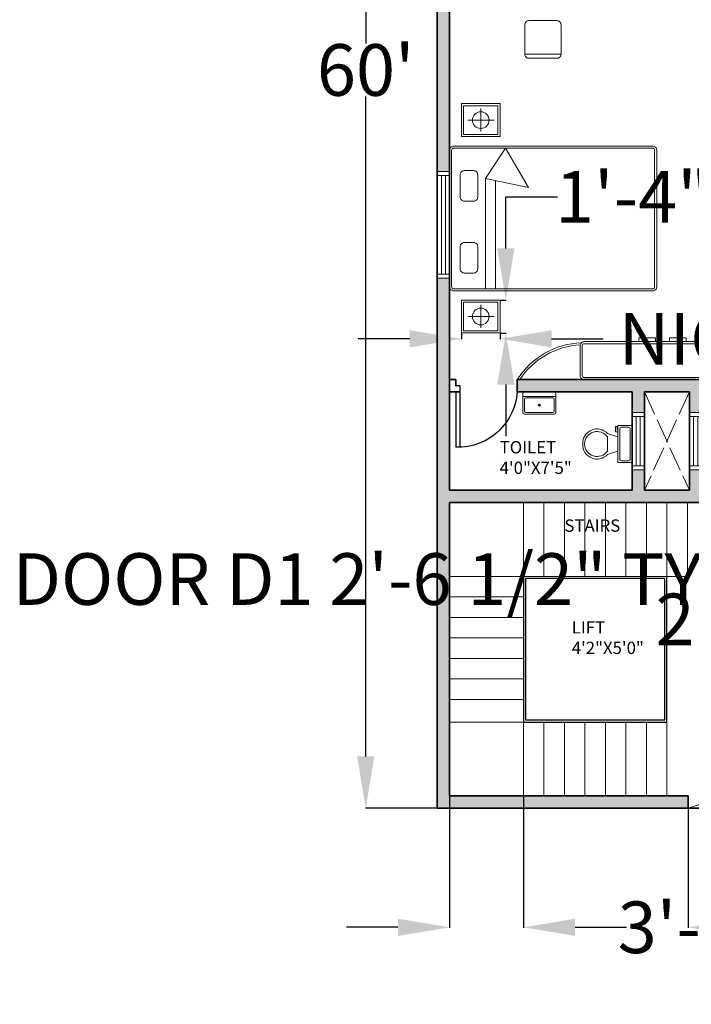
# Model space of a CAD drawing. Units: inches. Extents: x 35 to 5908, y 4 to 3165.
# Tile 1 of 6: x 4845 to 5173, y 2226 to 2706. Entities that reach past the tile are written whole.
import ezdxf

# ---------------------------------------------------------------- set-up
doc = ezdxf.new("R2010")
doc.units = ezdxf.units.IN
doc.header["$MEASUREMENT"] = 0
doc.linetypes.add('ACAD_ISO02W100', pattern=[15, 12, -3])
for name, color, linetype, lineweight in [('A-ANNO-DIMS', 2, 'Continuous', 18), ('A-ANNO-SYMB', 7, 'Continuous', 18), ('A-DOOR', 4, 'Continuous', 25), ('A-FLOR-CASE', 8, 'Continuous', 18), ('A-FLOR-EVTR', 7, 'Continuous', 25), ('A-FLOR-FIXT', 8, 'Continuous', 18), ('A-FLOR-SHFT', 8, 'ACAD_ISO02W100', 13), ('A-FLOR-STRS', 7, 'Continuous', 18), ('A-FURN', 8, 'Continuous', 18), ('A-WALL', 7, 'Continuous', 35), ('A-WALL-PATT', 252, 'Continuous', 13)]:
    doc.layers.add(name, color=color, linetype=linetype, lineweight=lineweight)
doc.layers.add('A-AREA-IDEN', color=30, linetype='Continuous', lineweight=18, true_color=0xf8991e)
doc.layers.add('A-GLAZ', color=30, linetype='Continuous', lineweight=18, true_color=0xf8991e)
doc.styles.get("Standard").update_dxf_attribs({"font": 'arial.ttf'})
doc.dimstyles.get("Standard").update_dxf_attribs({"dimtxt": 25.18, "dimasz": 25.18, "dimexe": 0.18, "dimexo": 0.0625, "dimgap": 0.09, "dimtad": 0, "dimtih": 1, "dimtoh": 1, "dimdec": 0, "dimzin": 0, "dimdsep": 46, "dimlunit": 3, "dimtxsty": 'Standard', "dimcen": 0.09, "dimadec": 0, "dimazin": 0, "dimtfac": 1, "dimtdec": 0, "dimtofl": 0, "dimtmove": 0, "dimatfit": 3, "dimfxl": 1, "dimtolj": 1, "dimtzin": 0, "dimarcsym": 0})

# ---------------------------------------------------------------- blocks, each defined once
blk = doc.blocks.new('Sink-single - 30 in top')
blk.add_line((-15, -3.999996), (15, -3.999996))
for points in [[(-13.5, 0), (13.5, 0)], [(-15, -18.499996), (-15, -1.5)], [(-13.5, -17.499996), (-13.5, -6.499996)], [(-12.5, -5.499996), (12.5, -5.499996)], [(13.5, -6.499996), (13.5, -17.499996)], [(15, -1.5), (15, -18.499996)], [(13.5, -19.999996), (-13.5, -19.999996)], [(12.5, -18.499996), (-12.5, -18.499996)]]:
    blk.add_lwpolyline(points)
for radius in [1, 0.5]:
    blk.add_circle((0, -11.999996), radius)
for centre, radius, start, end in [((-13.5, -1.5), 1.5, 90, 180), ((-12.5, -6.499996), 1, 90, 180), ((12.5, -6.499996), 1, 0, 90), ((13.5, -1.5), 1.5, 0, 90), ((-12.5, -17.499996), 1, 180, 270), ((12.5, -17.499996), 1, 270, 0), ((-13.5, -18.499996), 1.5, 180, 270), ((13.5, -18.499996), 1.5, 270, 0)]:
    blk.add_arc(centre, radius, start, end)
blk = doc.blocks.new('*U4')
for p, q in [((9.5, -6), (9.5, -2)), ((-10, -8.5), (-8, -8.5)), ((-10, -9.5), (-10, -8.5)), ((-7, -9.5), (-10, -9.5)), ((-8, -8.5), (-8, -8)), ((-7, -8), (-7, -9.5)), ((-4, -8), (-6, -14)), ((4, -8), (6, -14)), ((4, -14), (-4, -14))]:
    blk.add_line(p, q)
blk.add_lwpolyline([(10.5, -8), (10.5, 0), (-10.5, 0), (-10.5, -8)], close=True)
for points in [[(-9.5, -2), (-9.5, -6)], [(8.5, -1), (-8.5, -1)], [(-8.5, -7), (8.5, -7)]]:
    blk.add_lwpolyline(points)
for centre, radius, start, end in [((-8.625, -1.875), 0.8839, 81.8699, 188.1301), ((8.625, -1.875), 0.8839, 351.8699, 98.1301), ((-8.625, -6.125), 0.8839, 171.869898, 278.1301), ((8.625, -6.125), 0.8839, 261.8699, 8.1301), ((-0.4772, -19.9188), 8.0953, 133.01722, 273.38), ((0.0374, -19.8731), 7.127, 124.50543, 269.7), ((-0.0373, -19.8731), 7.127, 270.3, 55.4946), ((0.4773, -19.9188), 8.0953, 266.62, 46.9828)]:
    blk.add_arc(centre, radius, start, end)
blk = doc.blocks.new('*D7')
at = {"layer": 'A-ANNO-DIMS', "color": 0, "lineweight": -2, "transparency": 16777216}
for p, q in [((5048.73, 3041.84), (5013.71, 3041.84)), ((5013.89, 3016.66), (5013.89, 2694.76)), ((5013.89, 2346.96), (5013.89, 2668.86)), ((5048.73, 2321.78), (5013.71, 2321.78))]:
    blk.add_line(p, q, dxfattribs=at)
for points in [[(5009.69, 3016.66), (5018.09, 3016.66), (5013.89, 3041.84)], [(5009.69, 2346.96), (5018.09, 2346.96), (5013.89, 2321.78)]]:
    blk.add_solid(points, dxfattribs=at)
at = {"layer": 'Defpoints', "color": 0, "lineweight": -2, "transparency": 16777216}
for p in [(5048.79, 3041.84), (5013.89, 2321.78), (5048.79, 2321.78)]:
    blk.add_point(p, dxfattribs=at)
at = {"layer": 'A-ANNO-DIMS', "color": 0, "transparency": 16777216, "insert": (5013.89, 2681.81), "char_height": 25.18, "attachment_point": 5}
blk.add_mtext("\\A1;60'", dxfattribs=at)
blk = doc.blocks.new('DOOR-30-3-JAMB')
for p, q in [((-2, -27), (-2, 0)), ((0, -30), (0, 0)), ((0, -30), (-2, -30))]:
    blk.add_line(p, q)
blk.add_arc((-1, -29), 29.02, 358.0251, 91.9749)
blk = doc.blocks.new('WINDOW-48')
for p, q in [((0, 0), (0, 6)), ((2, 0), (2, 6)), ((50, 0), (50, 6)), ((52, 0), (52, 6)), ((2, 4), (50, 4)), ((2, 2), (50, 2))]:
    blk.add_line(p, q)
blk = doc.blocks.new('WINDOW-24')
for p, q in [((0, 0), (0, 6)), ((2, 0), (2, 6)), ((26, 0), (26, 6)), ((28, 0), (28, 6)), ((2, 4), (26, 4)), ((2, 2), (26, 2))]:
    blk.add_line(p, q)
blk = doc.blocks.new('NIGHTSTAND-RECT')
for p, q in [((0, 5.63), (0, -5.6)), ((-6.31, 0), (6.62, 0))]:
    blk.add_line(p, q)
for points in [[(-9.42, 8.04), (9.42, 8.04), (9.42, -8.04), (-9.42, -8.04)], [(-8.42, 7.04), (-8.42, 7.04), (8.42, 7.04), (8.42, 7.04), (8.42, -7.04), (8.42, -7.04), (-8.42, -7.04), (-8.42, -7.04)]]:
    blk.add_lwpolyline(points, close=True)
blk.add_circle((0, 0), 4.08)
blk = doc.blocks.new('*D26')
at = {"layer": 'A-ANNO-DIMS', "color": 0, "lineweight": -2, "transparency": 16777216}
for p, q in [((5241.11, 2433.5), (5215.93, 2433.5)), ((5266.29, 2429.02), (5266.29, 2433.68)), ((5296.57, 2429.02), (5296.57, 2433.68)), ((5321.75, 2433.5), (5346.93, 2433.5))]:
    blk.add_line(p, q, dxfattribs=at)
for points in [[(5241.11, 2437.7), (5241.11, 2429.3), (5266.29, 2433.5)], [(5321.75, 2437.7), (5321.75, 2429.3), (5296.57, 2433.5)]]:
    blk.add_solid(points, dxfattribs=at)
at = {"layer": 'Defpoints', "color": 0, "lineweight": -2, "transparency": 16777216}
for p in [(5266.29, 2433.5), (5266.29, 2428.96), (5296.57, 2428.96)]:
    blk.add_point(p, dxfattribs=at)
at = {"layer": 'A-ANNO-DIMS', "color": 0, "transparency": 16777216, "insert": (5025.37, 2433.5), "char_height": 25.18, "attachment_point": 5}
blk.add_mtext('\\A1;DOOR D1 2\'-6 1/2" TYP.', dxfattribs=at)
blk = doc.blocks.new('*D27')
at = {"layer": 'A-ANNO-DIMS', "color": 0, "lineweight": -2, "transparency": 16777216}
for p, q in [((5261.75, 2454.14), (5261.75, 2479.32)), ((5266.23, 2428.96), (5261.57, 2428.96)), ((5266.23, 2398.68), (5261.57, 2398.68)), ((5261.75, 2373.5), (5261.75, 2348.32))]:
    blk.add_line(p, q, dxfattribs=at)
for points in [[(5257.56, 2454.14), (5265.95, 2454.14), (5261.75, 2428.96)], [(5257.56, 2373.5), (5265.95, 2373.5), (5261.75, 2398.68)]]:
    blk.add_solid(points, dxfattribs=at)
at = {"layer": 'Defpoints', "color": 0, "lineweight": -2, "transparency": 16777216}
for p in [(5266.29, 2428.96), (5261.75, 2398.68), (5266.29, 2398.68)]:
    blk.add_point(p, dxfattribs=at)
at = {"layer": 'A-ANNO-DIMS', "color": 0, "transparency": 16777216, "insert": (5261.75, 2413.82), "char_height": 25.18, "attachment_point": 5}
blk.add_mtext('\\A1;2\'-6 1/2" TYP.', dxfattribs=at)
blk = doc.blocks.new('*D33')
at = {"layer": 'A-ANNO-DIMS', "color": 0, "lineweight": -2, "transparency": 16777216}
for p, q in [((5271.74, 2806.23), (5271.74, 2831.41)), ((5266.36, 2781.05), (5271.92, 2781.05)), ((5266.36, 2744.78), (5271.92, 2744.78)), ((5271.74, 2719.6), (5271.74, 2694.42))]:
    blk.add_line(p, q, dxfattribs=at)
for points in [[(5267.54, 2806.23), (5275.93, 2806.23), (5271.74, 2781.05)], [(5267.54, 2719.6), (5275.93, 2719.6), (5271.74, 2744.78)]]:
    blk.add_solid(points, dxfattribs=at)
at = {"layer": 'Defpoints', "color": 0, "lineweight": -2, "transparency": 16777216}
for p in [(5266.29, 2781.05), (5271.74, 2781.05), (5266.29, 2744.78)]:
    blk.add_point(p, dxfattribs=at)
at = {"layer": 'A-ANNO-DIMS', "color": 0, "transparency": 16777216, "insert": (5271.74, 2762.92), "char_height": 25.18, "attachment_point": 5}
blk.add_mtext('\\A1;3\'-0 1/2" TYP.', dxfattribs=at)
blk = doc.blocks.new('*D38')
at = {"layer": 'A-ANNO-DIMS', "color": 0, "lineweight": -2, "transparency": 16777216}
for p, q in [((5035.37, 2550.69), (5010.19, 2550.69)), ((5060.55, 2553.45), (5060.55, 2550.51)), ((5079.39, 2553.45), (5079.39, 2550.51)), ((5104.57, 2550.69), (5129.75, 2550.69))]:
    blk.add_line(p, q, dxfattribs=at)
for points in [[(5035.37, 2554.88), (5035.37, 2546.49), (5060.55, 2550.69)], [(5104.57, 2554.88), (5104.57, 2546.49), (5079.39, 2550.69)]]:
    blk.add_solid(points, dxfattribs=at)
at = {"layer": 'Defpoints', "color": 0, "lineweight": -2, "transparency": 16777216}
for p in [(5060.55, 2553.51), (5079.39, 2553.51), (5079.39, 2550.69)]:
    blk.add_point(p, dxfattribs=at)
at = {"layer": 'A-ANNO-DIMS', "color": 0, "transparency": 16777216, "insert": (5325.18, 2550.69), "char_height": 25.18, "attachment_point": 5}
blk.add_mtext('\\A1;NIGHTSTAND 1\'-7" TYP.', dxfattribs=at)
blk = doc.blocks.new('*D39')
at = {"layer": 'A-ANNO-DIMS', "color": 0, "lineweight": -2, "transparency": 16777216}
for p, q in [((5082.21, 2594.78), (5082.21, 2619.96)), ((5082.21, 2619.96), (5107.39, 2619.96)), ((5079.45, 2569.6), (5082.39, 2569.6)), ((5079.45, 2553.51), (5082.39, 2553.51)), ((5082.21, 2528.33), (5082.21, 2503.15))]:
    blk.add_line(p, q, dxfattribs=at)
for points in [[(5078.01, 2594.78), (5086.41, 2594.78), (5082.21, 2569.6)], [(5078.01, 2528.33), (5086.41, 2528.33), (5082.21, 2553.51)]]:
    blk.add_solid(points, dxfattribs=at)
at = {"layer": 'Defpoints', "color": 0, "lineweight": -2, "transparency": 16777216}
for p in [(5079.39, 2569.6), (5082.21, 2569.6), (5079.39, 2553.51)]:
    blk.add_point(p, dxfattribs=at)
at = {"layer": 'A-ANNO-DIMS', "color": 0, "transparency": 16777216, "insert": (5183.04, 2619.96), "char_height": 25.18, "attachment_point": 5}
blk.add_mtext('\\A1;1\'-4" TYP.', dxfattribs=at)
blk = doc.blocks.new('*D48')
at = {"layer": 'A-ANNO-DIMS', "color": 0, "lineweight": -2, "transparency": 16777216}
for p, q in [((5054.79, 2327.72), (5054.79, 2263.46)), ((5090.79, 2327.72), (5090.79, 2263.46)), ((5029.61, 2263.64), (5004.43, 2263.64)), ((5115.97, 2263.64), (5141.15, 2263.64))]:
    blk.add_line(p, q, dxfattribs=at)
for points in [[(5029.61, 2267.83), (5029.61, 2259.44), (5054.79, 2263.64)], [(5115.97, 2267.83), (5115.97, 2259.44), (5090.79, 2263.64)]]:
    blk.add_solid(points, dxfattribs=at)
at = {"layer": 'Defpoints', "color": 0, "lineweight": -2, "transparency": 16777216}
for p in [(5054.79, 2327.78), (5090.79, 2327.78), (5090.79, 2263.64)]:
    blk.add_point(p, dxfattribs=at)
at = {"layer": 'A-ANNO-DIMS', "color": 0, "transparency": 16777216, "insert": (5174.7, 2263.64), "char_height": 25.18, "attachment_point": 5}
blk.add_mtext('\\A1;3\'-0"', dxfattribs=at)
blk = doc.blocks.new('*D49')
at = {"layer": 'A-ANNO-DIMS', "color": 0, "lineweight": -2, "transparency": 16777216}
for p, q in [((5171.13, 2321.72), (5171.13, 2263.46)), ((5262.79, 2321.72), (5262.79, 2263.46)), ((5196.31, 2263.64), (5237.61, 2263.64)), ((5262.79, 2263.64), (5287.97, 2263.64))]:
    blk.add_line(p, q, dxfattribs=at)
for points in [[(5196.31, 2267.83), (5196.31, 2259.44), (5171.13, 2263.64)], [(5237.61, 2267.83), (5237.61, 2259.44), (5262.79, 2263.64)]]:
    blk.add_solid(points, dxfattribs=at)
at = {"layer": 'Defpoints', "color": 0, "lineweight": -2, "transparency": 16777216}
for p in [(5171.13, 2321.78), (5262.79, 2321.78), (5262.79, 2263.64)]:
    blk.add_point(p, dxfattribs=at)
at = {"layer": 'A-ANNO-DIMS', "color": 0, "transparency": 16777216, "insert": (5350.77, 2263.64), "char_height": 25.18, "attachment_point": 5}
blk.add_mtext('\\A1;7\'-7 1/2"', dxfattribs=at)

msp = doc.modelspace()

# ---------------------------------------------------------------- hatches: boundary and pattern name
at = {"layer": 'A-WALL-PATT'}
h = msp.add_hatch(color=256, dxfattribs=at)
h.dxf.hatch_style = 1
h.paths.add_polyline_path([(5198.29, 3041.78), (5119.29, 3041.78), (5119.29, 3035.78), (5155.79, 3035.78), (5155.79, 2967.78), (5087.79, 2967.78), (5087.79, 2966.78, -0.017236), (5087.79, 2964.78), (5087.79, 2961.78), (5262.79, 2961.78), (5262.79, 2967.78), (5236.55, 2967.78), (5236.55, 2967.75), (5218.53, 2967.75), (5161.79, 2967.78), (5161.79, 3035.78), (5198.29, 3035.78)])
h.paths.add_polyline_path([(5091.29, 3041.78), (5048.79, 3041.78), (5048.79, 2877.78), (5054.79, 2877.78), (5054.79, 2899), (5054.79, 2961.78), (5054.79, 2967.78), (5054.79, 3035.78), (5091.29, 3035.78)])
h.paths.add_polyline_path([(5346.29, 3041.78), (5226.29, 3041.78), (5226.29, 3035.78), (5262.79, 3035.78), (5269.79, 3035.78), (5346.29, 3035.78)])
h.paths.add_polyline_path([(5480.79, 3041.78), (5398.29, 3041.78), (5398.29, 3035.78), (5407.91, 3035.78), (5474.79, 3035.78), (5474.79, 2807.78), (5269.79, 2807.78), (5269.79, 3002.78), (5266.29, 3002.78, -0.017236), (5264.29, 3002.78), (5262.79, 3002.78), (5262.79, 2967.78), (5262.79, 2961.78), (5262.79, 2780.78), (5264.29, 2780.78, -0.014283), (5266.29, 2780.78), (5269.79, 2780.78), (5269.79, 2801.78), (5412.79, 2801.78), (5412.79, 2712.78), (5346.79, 2712.78), (5346.79, 2706.78), (5421.79, 2706.78), (5421.79, 2709.78, -0.017236), (5421.79, 2711.78), (5421.79, 2712.78), (5418.79, 2712.78), (5418.79, 2801.78), (5474.79, 2801.78), (5474.79, 2712.78), (5454.79, 2712.78), (5454.79, 2706.78), (5474.79, 2706.78), (5474.79, 2668.42), (5480.79, 2668.42)])
h.paths.add_polyline_path([(5054.79, 2825.78), (5048.79, 2825.78), (5048.79, 2632.28), (5054.79, 2632.28), (5054.79, 2642.69), (5054.79, 2735.78), (5262.79, 2735.78), (5262.79, 2741.78), (5054.79, 2741.78)])
h.paths.add_polyline_path([(5480.79, 2616.42), (5474.79, 2616.42), (5474.79, 2502.2), (5480.79, 2502.2)])
h.paths.add_polyline_path([(5407.53, 2562.78), (5269.79, 2562.78), (5269.79, 2696.78), (5266.29, 2696.78, -0.014283), (5264.29, 2696.78), (5262.79, 2696.78), (5262.79, 2509.78), (5264.29, 2509.78, -0.017236), (5266.29, 2509.78), (5269.79, 2509.78), (5269.79, 2556.78), (5407.53, 2556.78)])
h.paths.add_polyline_path([(5262.79, 2530.78), (5087.79, 2530.78), (5087.79, 2527.78, -0.017236), (5087.79, 2525.78), (5087.79, 2524.78), (5143.79, 2524.78), (5143.79, 2514.78), (5149.79, 2514.78), (5149.79, 2524.78), (5171.79, 2524.78), (5171.79, 2514.78), (5177.79, 2514.78), (5177.79, 2524.78), (5262.79, 2524.78)], flags=17)
h.paths.add_polyline_path([(5262.79, 2395.71), (5262.79, 2321.78), (5480.79, 2321.78), (5480.79, 2450.2), (5474.79, 2450.2), (5474.79, 2381.78), (5425.29, 2381.78), (5425.29, 2375.78), (5474.79, 2375.78), (5474.79, 2327.78), (5269.79, 2327.78), (5269.79, 2375.78), (5312.61, 2375.78), (5312.61, 2381.78), (5269.79, 2381.78), (5269.79, 2395.71)])
h.paths.add_polyline_path([(5171.13, 2321.78), (5171.13, 2327.78), (5054.79, 2327.78), (5054.79, 2470.78), (5157.79, 2470.78), (5262.79, 2470.78), (5262.79, 2461.71), (5269.79, 2461.71), (5269.79, 2476.78), (5262.79, 2476.78), (5177.79, 2476.78), (5177.79, 2486.78), (5171.79, 2486.78), (5171.79, 2476.78), (5149.79, 2476.78), (5149.79, 2486.78), (5143.79, 2486.78), (5143.79, 2476.78), (5054.79, 2476.78), (5054.79, 2580.28), (5048.79, 2580.28), (5048.79, 2321.78)])

# ---------------------------------------------------------------- linework, layer by layer
at = {"layer": 'A-ANNO-SYMB'}
msp.add_open_spline([(5171.13, 2321.78), (5182.06, 2325.26), (5201.09, 2331.32), (5190.06, 2279.32), (5222.38, 2375.47), (5241.98, 2295.8), (5241.68, 2325.16), (5253.78, 2321.34), (5259.7, 2321.63), (5262.79, 2321.78)], degree=3, knots=[0, 0, 0, 0, 24.730916, 43.022674, 87.561703, 119.186713, 129.816728, 138.741517, 148.526637, 148.526637, 148.526637, 148.526637], dxfattribs=at)
at = {"layer": 'A-FLOR-CASE'}
for points in [[(5147.17, 2549.31), (5147.17, 2549.31), (5155.25, 2549.31), (5155.25, 2549.31), (5155.25, 2551.08), (5155.25, 2551.08), (5147.17, 2551.08), (5147.17, 2551.08)], [(5162.1, 2549.31), (5162.1, 2549.31), (5170.18, 2549.31), (5170.18, 2549.31), (5170.18, 2551.08), (5170.18, 2551.08), (5162.1, 2551.08), (5162.1, 2551.08)]]:
    msp.add_lwpolyline(points, close=True, dxfattribs=at)
for points in [[(5262.79, 2532.78, -0.414214), (5260.79, 2530.78), (5120.49, 2530.78, -0.414214), (5118.49, 2532.78), (5118.49, 2547.31, -0.414214), (5120.49, 2549.31), (5260.79, 2549.31, -0.414214), (5262.79, 2547.31)], [(5261.79, 2532.78, -0.414214), (5260.79, 2531.78), (5120.49, 2531.78, -0.414214), (5119.49, 2532.78), (5119.49, 2547.31, -0.414214), (5120.49, 2548.31), (5260.79, 2548.31, -0.414214), (5261.79, 2547.31)]]:
    msp.add_lwpolyline(points, format="xyb", close=True, dxfattribs=at)
for radius, start, end in [(38.5, 91.91, 147.7627), (37.5, 92.7978, 146.7939)]:
    msp.add_arc((5120.36, 2510.24), radius, start, end, dxfattribs=at)
at = {"layer": 'A-FLOR-EVTR'}
for p, q in [((5090.79, 2434.78), (5090.79, 2363.78)), ((5091.79, 2433.78), (5091.79, 2364.78)), ((5159.79, 2433.78), (5091.79, 2433.78)), ((5159.79, 2364.78), (5159.79, 2433.78)), ((5160.79, 2363.78), (5160.79, 2434.78)), ((5090.79, 2363.78), (5160.79, 2363.78)), ((5091.79, 2364.78), (5159.79, 2364.78))]:
    msp.add_line(p, q, dxfattribs=at)
at = {"layer": 'A-FLOR-SHFT'}
for p, q in [((5149.79, 2524.78), (5171.79, 2476.78)), ((5171.79, 2524.78), (5149.79, 2476.78))]:
    msp.add_line(p, q, dxfattribs=at)
at = {"layer": 'A-FLOR-STRS'}
for p, q in [((5090.79, 2327.78), (5090.79, 2470.78)), ((5100.79, 2434.78), (5100.79, 2470.78)), ((5110.79, 2434.78), (5110.79, 2470.78)), ((5120.79, 2434.78), (5120.79, 2470.78)), ((5130.79, 2434.78), (5130.79, 2470.78)), ((5140.79, 2434.78), (5140.79, 2470.78)), ((5150.79, 2434.78), (5150.79, 2470.78)), ((5160.79, 2434.78), (5160.79, 2470.78)), ((5170.79, 2434.78), (5170.79, 2470.78)), ((5170.79, 2434.78), (5054.79, 2434.78)), ((5090.79, 2424.78), (5054.79, 2424.78)), ((5090.79, 2414.78), (5054.79, 2414.78)), ((5090.79, 2404.78), (5054.79, 2404.78)), ((5090.79, 2394.78), (5054.79, 2394.78)), ((5090.79, 2384.78), (5054.79, 2384.78)), ((5090.79, 2374.78), (5054.79, 2374.78)), ((5160.79, 2363.78), (5054.79, 2363.78)), ((5100.79, 2327.78), (5100.79, 2363.78)), ((5110.79, 2327.78), (5110.79, 2363.78)), ((5120.79, 2327.78), (5120.79, 2363.78)), ((5130.79, 2327.78), (5130.79, 2363.78)), ((5140.79, 2327.78), (5140.79, 2363.78)), ((5150.79, 2327.78), (5150.79, 2363.78)), ((5160.79, 2327.78), (5160.79, 2363.78))]:
    msp.add_line(p, q, dxfattribs=at)
at = {"layer": 'A-FURN'}
for p, q in [((5091.48, 2689.49), (5109.13, 2689.49)), ((5072.24, 2628.84), (5082.1, 2643.69)), ((5082.1, 2643.69), (5093.21, 2624.46)), ((5072.24, 2575.02), (5072.24, 2628.84)), ((5093.21, 2624.46), (5072.24, 2628.84)), ((5077.12, 2627.82), (5077.12, 2575.02))]:
    msp.add_line(p, q, dxfattribs=at)
for points in [[(5091.48, 2703.89, -0.414214), (5093.48, 2705.89), (5107.13, 2705.89, -0.414214), (5109.13, 2703.89), (5109.13, 2689.49, -0.414214), (5107.13, 2687.49), (5093.48, 2687.49, -0.414214), (5091.48, 2689.49)], [(5054.79, 2576.02, 0.414214), (5056.79, 2574.02), (5153.81, 2574.02, 0.414214), (5155.81, 2576.02), (5155.81, 2642.69, 0.414214), (5153.81, 2644.69), (5056.79, 2644.69, 0.414214), (5054.79, 2642.69)], [(5055.79, 2576.02, 0.414214), (5056.79, 2575.02), (5153.81, 2575.02, 0.414214), (5154.81, 2576.02), (5154.81, 2642.69, 0.414214), (5153.81, 2643.69), (5056.79, 2643.69, 0.414214), (5055.79, 2642.69)], [(5059.95, 2630.72, -0.414214), (5061.95, 2632.72), (5066.5, 2632.72, -0.414214), (5068.5, 2630.72), (5068.5, 2619.82, -0.414214), (5066.5, 2617.82), (5061.95, 2617.82, -0.414214), (5059.95, 2619.82)], [(5059.95, 2595.67, -0.414214), (5061.95, 2597.67), (5066.5, 2597.67, -0.414214), (5068.5, 2595.67), (5068.5, 2584.78, -0.414214), (5066.5, 2582.78), (5061.95, 2582.78, -0.414214), (5059.95, 2584.78)]]:
    msp.add_lwpolyline(points, format="xyb", close=True, dxfattribs=at)
at = {"layer": 'A-WALL'}
for p, q in [((5048.79, 2321.78), (5048.79, 3041.78)), ((5054.79, 2476.78), (5054.79, 2735.78)), ((5057.79, 2530.78), (5054.79, 2530.78)), ((5057.79, 2527.78), (5057.79, 2530.78)), ((5262.79, 2530.78), (5087.79, 2530.78)), ((5087.79, 2524.78), (5087.79, 2530.78)), ((5059.79, 2524.78), (5054.79, 2524.78)), ((5143.79, 2524.78), (5087.74, 2524.78)), ((5143.79, 2476.78), (5143.79, 2524.78)), ((5149.79, 2476.78), (5149.79, 2524.78)), ((5171.79, 2524.78), (5149.79, 2524.78)), ((5171.79, 2476.78), (5171.79, 2524.78)), ((5143.79, 2476.78), (5054.79, 2476.78)), ((5171.79, 2476.78), (5149.79, 2476.78)), ((5054.79, 2327.78), (5054.79, 2470.78)), ((5262.79, 2470.78), (5054.79, 2470.78)), ((5157.79, 2470.78), (5054.79, 2470.78)), ((5171.13, 2327.78), (5054.79, 2327.78)), ((5171.13, 2327.78), (5171.13, 2321.78)), ((5171.13, 2321.78), (5048.79, 2321.78)), ((5171.13, 2321.78), (5262.79, 2321.78))]:
    msp.add_line(p, q, dxfattribs=at)

# ---------------------------------------------------------------- block references
at = {"layer": 'A-DOOR', "extrusion": (0, 0, -1), "zscale": -1, "rotation": 180}
msp.add_blockref('DOOR-30-3-JAMB', (-5059.79, 2497.78), dxfattribs=at)
at = {"layer": 'A-FLOR-FIXT', "xscale": 0.5392550146415948, "yscale": 0.5392550146415948, "zscale": 0.5392550146415948}
msp.add_blockref('Sink-single - 30 in top', (5098.58, 2524.78), dxfattribs=at)
at = {"layer": 'A-FLOR-FIXT', "xscale": 0.8581878397813429, "yscale": 0.8581878397813429, "zscale": 0.8581878397813429, "rotation": 270}
msp.add_blockref('*U4', (5143.79, 2499.37), dxfattribs=at)
at = {"layer": 'A-FURN'}
for p in [(5069.97, 2657.35), (5069.97, 2561.56)]:
    msp.add_blockref('NIGHTSTAND-RECT', p, dxfattribs=at)
at = {"layer": 'A-GLAZ'}
for name, p, rotation in [('WINDOW-48', (5054.79, 2580.28), 90.0000000000016), ('WINDOW-24', (5143.79, 2514.78), 269.999999999994), ('WINDOW-24', (5171.79, 2514.78), 270.0000000000012)]:
    msp.add_blockref(name, p, dxfattribs=dict(at, rotation=rotation))

# ---------------------------------------------------------------- texts
at = {"layer": 'A-AREA-IDEN', "char_height": 6, "attachment_point": 1}
for s, insert in [('TOILET\\P4\'0"X7\'5"', (5079.22, 2500.78)), ('STAIRS', (5110.79, 2462.59)), ('LIFT\\P4\'2"X5\'0"', (5114.38, 2412.95))]:
    msp.add_mtext_dynamic_manual_height_columns(s, width=69.8687, gutter_width=1, heights=[0], dxfattribs=dict(at, insert=insert))

# ---------------------------------------------------------------- dimensions: what is measured, and where the dimension line sits
at = {"layer": 'A-ANNO-DIMS'}
dim = msp.add_linear_dim(base=(5013.89, 2321.78), p1=(5048.79, 3041.84), p2=(5048.79, 2321.78), angle=90, dimstyle='Standard', override={"dimclrd": 0, "dimclre": 0, "dimclrt": 0}, dxfattribs=at)
dim.commit()
dim.dimension.update_dxf_attribs({"geometry": '*D7', "text_midpoint": (5013.89, 2681.81)})
for base, p1, p2, angle, text, picture, middle in [((5271.74, 2781.05), (5266.29, 2744.78), (5266.29, 2781.05), 90, '<> TYP.', '*D33', (5271.74, 2762.92)), ((5082.21, 2569.6), (5079.39, 2553.51), (5079.39, 2569.6), 90, '<> TYP.', '*D39', (5183.04, 2619.96)), ((5266.29, 2433.5), (5296.57, 2428.96), (5266.29, 2428.96), 180, 'DOOR D1 <> TYP.', '*D26', (5025.37, 2433.5)), ((5261.75, 2398.68), (5266.29, 2428.96), (5266.29, 2398.68), 270, '<> TYP.', '*D27', (5261.75, 2413.82))]:
    dim = msp.add_linear_dim(base=base, p1=p1, p2=p2, angle=angle, text=text, dimstyle='Standard', override={"dimdec": 1, "dimlfac": 1, "dimrnd": 0, "dimzin": 1, "dimdsep": 46, "dimlunit": 4, "dimfrac": 2}, dxfattribs=at)
    dim.commit()
    dim.dimension.update_dxf_attribs({"geometry": picture, "text_midpoint": middle})
dim = msp.add_linear_dim(base=(5079.39, 2550.69), p1=(5060.55, 2553.51), p2=(5079.39, 2553.51), text='NIGHTSTAND <> TYP.', dimstyle='Standard', override={"dimdec": 1, "dimlfac": 1, "dimrnd": 0, "dimzin": 1, "dimdsep": 46, "dimlunit": 4, "dimfrac": 2}, dxfattribs=at)
dim.commit()
dim.dimension.update_dxf_attribs({"geometry": '*D38', "text_midpoint": (5325.18, 2550.69)})
for base, p1, p2, picture, middle in [((5090.79, 2263.64), (5054.79, 2327.78), (5090.79, 2327.78), '*D48', (5174.7, 2263.64)), ((5262.79, 2263.64), (5171.13, 2321.78), (5262.79, 2321.78), '*D49', (5350.77, 2263.64))]:
    dim = msp.add_linear_dim(base=base, p1=p1, p2=p2, dimstyle='Standard', override={"dimdec": 1, "dimlfac": 1, "dimrnd": 0, "dimzin": 1, "dimdsep": 46, "dimlunit": 4, "dimfrac": 2}, dxfattribs=at)
    dim.commit()
    dim.dimension.update_dxf_attribs({"geometry": picture, "text_midpoint": middle})

doc.saveas('drawing.dxf')
